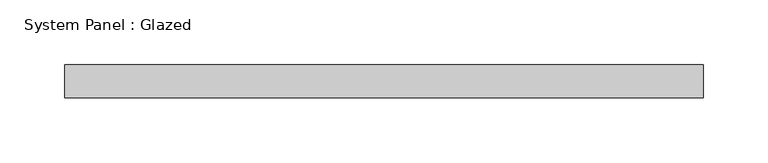
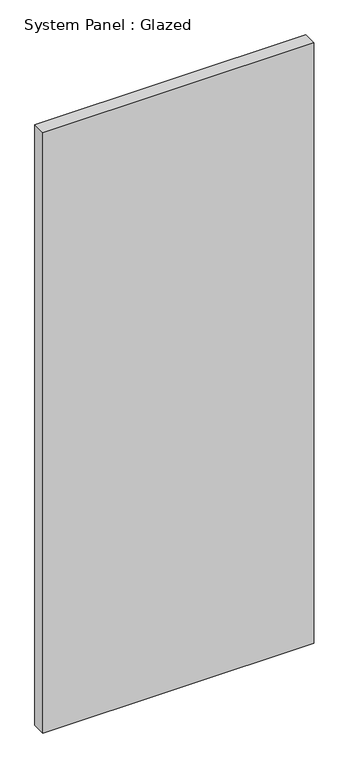
"""IFC4 building model written with IfcOpenShell, lengths in millimetres: plate geometry, System Panel : Glazed."""

from ifc_helpers import new_model, si_unit, origin, origin_with_axes, place, context, project, spatial, polyline, outline, extrude, source, transform, mapped, element, save


def system_panel_glazed_3daf8e53(model_context):
    return source(origin(), model_context, "Body", "SweptSolid", [
        extrude(outline(polyline([(246.4161825, 19.05), (-246.4161825, 19.05), (-246.4161825, 44.45), (246.4161825, 44.45), (246.4161825, 19.05)])), origin_with_axes(), (0.0, 0.0, 1.0), 1155.7),
    ])


if __name__ == "__main__":
    model = new_model("IFC4")
    model_context = context("Model", 3, world=origin())
    ifc_project = project(units=[si_unit("LENGTHUNIT", "METRE", prefix="MILLI")], contexts=[model_context])
    site = spatial("IfcSite", under=ifc_project)
    building = spatial("IfcBuilding", under=site)
    placement = place(None, origin())
    system_panel_glazed_shape = system_panel_glazed_3daf8e53(model_context)
    element("IfcPlate", 1, ObjectType="System Panel : Glazed", at=placement, inside=building, context=model_context, shape_type="MappedRepresentation", body=[
        mapped(system_panel_glazed_shape, transform((0.0, 0.0, 0.0), x_axis=(1.0, 0.0, 0.0), y_axis=(0.0, 1.0, 0.0), z_axis=(0.0, 0.0, 1.0))),
    ])
    save(model, "model.ifc")

# Revit data of these elements
# Type "System Panel : Glazed"
#   Construction Type Id = "GSP4R"
#   Analytic Construction = "1/8 in Pilkington single glazing"
#   Visual Light Transmittance = 0.9
#   Solar Heat Gain Coefficient = 0.86
#   Heat Transfer Coefficient (U) = 1.18115 BTU/(h·ft²·°F)
# Element 1 (IfcPlate, "System Panel : Glazed")
#   Materials on its faces: "Glass"
# Materials
#   "Glass": class "Glass", colour RGB 0 128 192, transparency 0.75, Description = "Soda Lime Glass", Cost = 0
